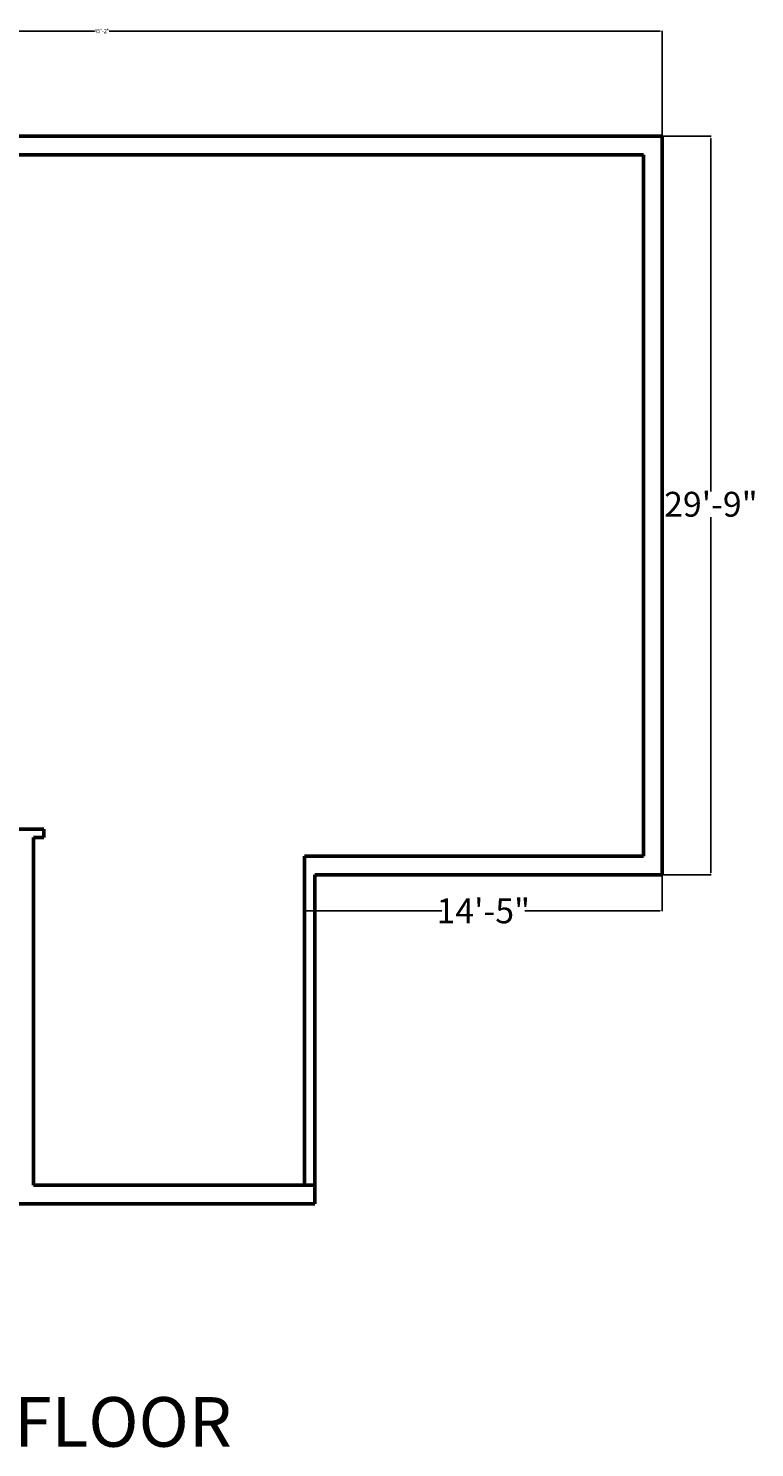
# Model space of a CAD drawing. Units: inches. Extents: x 409 to 7572, y 7 to 725.
# Tile 38 of 38: x 7221 to 7572, y 39 to 725. Entities that reach past the tile are written whole.
import ezdxf

# ---------------------------------------------------------------- set-up
doc = ezdxf.new("R2010")
doc.units = ezdxf.units.IN
doc.header["$MEASUREMENT"] = 0
for name, color, linetype, lineweight in [('A-ANNO-DIMS', 2, 'Continuous', 18), ('A-ANNO-TEXT', 7, 'Continuous', 35), ('A-WALL', 7, 'Continuous', 50)]:
    doc.layers.add(name, color=color, linetype=linetype, lineweight=lineweight)
doc.styles.get("Standard").update_dxf_attribs({"font": 'arial.ttf'})
doc.dimstyles.get("Standard").update_dxf_attribs({"dimtxt": 2, "dimasz": 1, "dimexe": 0.18, "dimexo": 0.0625, "dimgap": 0.09, "dimtad": 0, "dimtih": 1, "dimtoh": 1, "dimdec": 0, "dimzin": 0, "dimdsep": 46, "dimlunit": 3, "dimtxsty": 'Standard', "dimcen": 0.09, "dimadec": 0, "dimazin": 0, "dimtfac": 1, "dimtdec": 0, "dimtofl": 0, "dimtmove": 0, "dimatfit": 3, "dimfxl": 1, "dimtolj": 1, "dimtzin": 0, "dimarcsym": 0})

# ---------------------------------------------------------------- blocks, each defined once
blk = doc.blocks.new('*D161')
at = {"layer": 'A-ANNO-DIMS', "color": 0, "lineweight": -2, "transparency": 16777216}
for p, q in [((6985.41, 672.59), (6985.41, 723.56)), ((6986.41, 723.38), (7252.85, 723.38)), ((7526.41, 723.38), (7259.98, 723.38)), ((7527.41, 672.59), (7527.41, 723.56))]:
    blk.add_line(p, q, dxfattribs=at)
at = {"layer": 'A-ANNO-DIMS', "color": 0, "transparency": 16777216}
for points in [[(6986.41, 723.55), (6986.41, 723.22), (6985.41, 723.38)], [(7526.41, 723.55), (7526.41, 723.22), (7527.41, 723.38)]]:
    blk.add_solid(points, dxfattribs=at)
at = {"layer": 'DEFPOINTS', "color": 0, "transparency": 16777216}
for p in [(6985.41, 723.38), (6985.41, 672.53), (7527.41, 672.53)]:
    blk.add_point(p, dxfattribs=at)
at = {"layer": 'A-ANNO-DIMS', "color": 0, "transparency": 16777216, "insert": (7256.41, 723.38), "char_height": 2, "attachment_point": 5}
blk.add_mtext('\\A1;45\'-2"', dxfattribs=at)
blk = doc.blocks.new('*D163')
at = {"layer": 'A-ANNO-DIMS', "color": 0, "lineweight": -2, "transparency": 16777216}
for p, q in [((7527.47, 672.53), (7551.16, 672.53)), ((7550.98, 671.53), (7550.98, 500.86)), ((7550.98, 316.53), (7550.98, 488.43)), ((7527.47, 315.53), (7551.16, 315.53))]:
    blk.add_line(p, q, dxfattribs=at)
at = {"layer": 'A-ANNO-DIMS', "color": 0, "transparency": 16777216}
for points in [[(7550.81, 671.53), (7551.15, 671.53), (7550.98, 672.53)], [(7550.81, 316.53), (7551.15, 316.53), (7550.98, 315.53)]]:
    blk.add_solid(points, dxfattribs=at)
at = {"layer": 'DEFPOINTS', "color": 0, "transparency": 16777216}
for p in [(7527.41, 672.53), (7550.98, 672.53), (7527.41, 315.53)]:
    blk.add_point(p, dxfattribs=at)
at = {"layer": 'A-ANNO-DIMS', "color": 0, "transparency": 16777216, "insert": (7550.98, 494.65), "char_height": 2, "attachment_point": 5}
blk.add_mtext('\\A1;{\\H6x;29\'-9"}', dxfattribs=at)
blk = doc.blocks.new('*D162')
at = {"layer": 'A-ANNO-DIMS', "color": 0, "lineweight": -2, "transparency": 16777216}
for p, q in [((7354.41, 315.37), (7354.41, 297.9)), ((7527.41, 315.37), (7527.41, 297.9)), ((7355.41, 298.08), (7420.78, 298.08)), ((7526.41, 298.08), (7461.05, 298.08))]:
    blk.add_line(p, q, dxfattribs=at)
at = {"layer": 'A-ANNO-DIMS', "color": 0, "transparency": 16777216}
for points in [[(7355.41, 298.25), (7355.41, 297.92), (7354.41, 298.08)], [(7526.41, 298.25), (7526.41, 297.92), (7527.41, 298.08)]]:
    blk.add_solid(points, dxfattribs=at)
at = {"layer": 'DEFPOINTS', "color": 0, "transparency": 16777216}
for p in [(7354.41, 315.43), (7527.41, 315.43), (7527.41, 298.08)]:
    blk.add_point(p, dxfattribs=at)
at = {"layer": 'A-ANNO-DIMS', "color": 0, "transparency": 16777216, "insert": (7440.91, 298.08), "char_height": 2, "attachment_point": 5}
blk.add_mtext('\\A1;{\\H6x;14\'-5"}', dxfattribs=at)

msp = doc.modelspace()

# ---------------------------------------------------------------- linework, layer by layer
at = {"layer": 'A-WALL'}
for p, q in [((7527.41, 672.53), (6985.41, 672.53)), ((7527.41, 315.53), (7527.41, 672.53)), ((7518.41, 663.53), (7162.41, 663.53)), ((7518.41, 324.53), (7518.41, 663.53)), ((7518.41, 627.53), (7518.41, 663.53)), ((7518.41, 453.53), (7518.41, 489.53)), ((7518.41, 324.53), (7518.41, 444.53)), ((7207.41, 337.53), (7228.41, 337.53)), ((7228.41, 333.53), (7228.41, 337.53)), ((7223.41, 333.53), (7228.41, 333.53)), ((7223.41, 333.53), (7223.41, 165.53)), ((7518.41, 324.53), (7354.41, 324.53)), ((7354.41, 324.53), (7354.41, 165.53)), ((7354.41, 324.53), (7354.41, 165.53)), ((7527.41, 315.53), (7359.41, 315.53)), ((7359.41, 315.53), (7359.41, 165.53)), ((7223.41, 165.53), (7359.41, 165.53)), ((7359.41, 165.53), (7359.41, 156.53)), ((6985.41, 156.53), (7359.41, 156.53))]:
    msp.add_line(p, q, dxfattribs=at)

# ---------------------------------------------------------------- texts
at = {"layer": 'A-ANNO-TEXT', "insert": (7117.54, 63.03), "char_height": 24, "attachment_point": 1}
msp.add_mtext_dynamic_manual_height_columns('FIFTH FLOOR', width=577.2242, gutter_width=1, heights=[0], dxfattribs=at)

# ---------------------------------------------------------------- dimensions: what is measured, and where the dimension line sits
at = {"layer": 'A-ANNO-DIMS'}
dim = msp.add_linear_dim(base=(6985.41, 723.38), p1=(7527.41, 672.53), p2=(6985.41, 672.53), dimstyle='Standard', override={"dimclrd": 0, "dimclre": 0, "dimclrt": 0}, dxfattribs=at)
dim.commit()
dim.dimension.update_dxf_attribs({"geometry": '*D161', "text_midpoint": (7256.41, 723.38)})
dim = msp.add_linear_dim(base=(7550.98, 672.53), p1=(7527.41, 315.53), p2=(7527.41, 672.53), angle=90, text='{\\H6x;<>}', dimstyle='Standard', override={"dimclrd": 0, "dimclre": 0, "dimclrt": 0}, dxfattribs=at)
dim.commit()
dim.dimension.update_dxf_attribs({"geometry": '*D163', "text_midpoint": (7550.98, 494.65), "dimtype": 160})
dim = msp.add_linear_dim(base=(7527.41, 298.08), p1=(7354.41, 315.43), p2=(7527.41, 315.43), text='{\\H6x;<>}', dimstyle='Standard', override={"dimclrd": 0, "dimclre": 0, "dimclrt": 0}, dxfattribs=at)
dim.commit()
dim.dimension.update_dxf_attribs({"geometry": '*D162', "text_midpoint": (7440.91, 298.08)})

doc.saveas('drawing.dxf')
